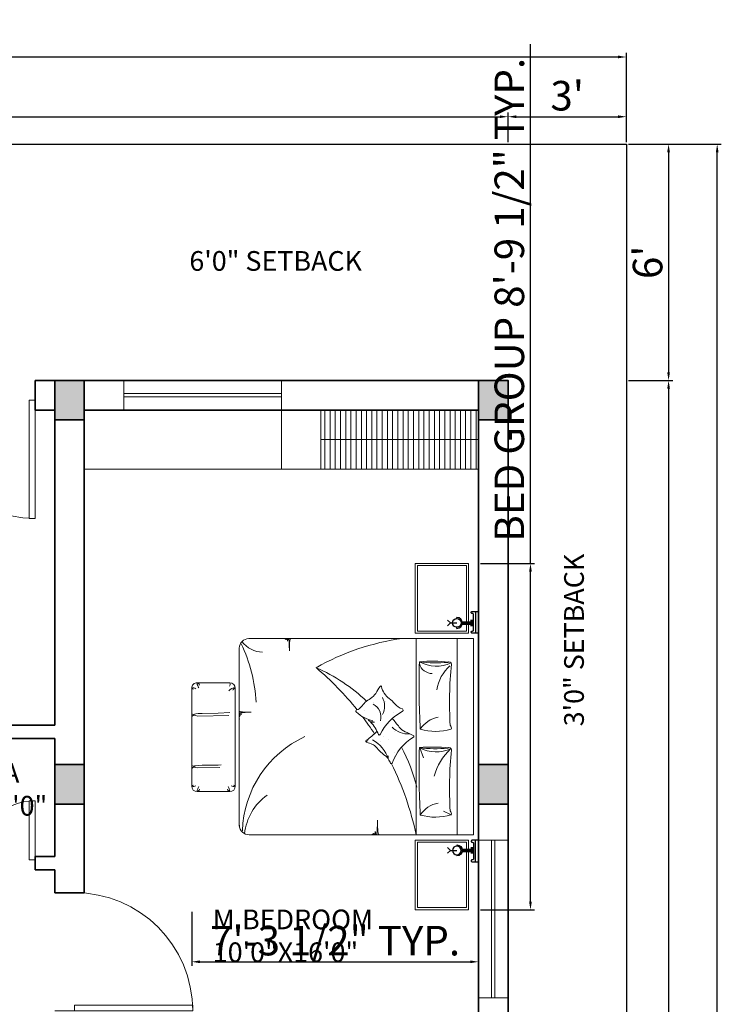
# Model space of a CAD drawing. Units: inches. Extents: x 3321 to 5237, y 11 to 1752.
# Tile 12 of 43: x 3652 to 3866, y 1445 to 1745. Entities that reach past the tile are written whole.
import ezdxf

# ---------------------------------------------------------------- set-up
doc = ezdxf.new("R2010")
doc.units = ezdxf.units.IN
for name, color, linetype, lineweight in [('A-ANNO-DIMS', 2, 'Continuous', 18), ('A-ANNO-TEXT', 7, 'Continuous', 18), ('A-AREA-IDEN', 7, 'Continuous', 18), ('A-COLS', 1, 'Continuous', 35), ('A-DOOR', 4, 'Continuous', 18), ('A-FLOR-CASE', 8, 'Continuous', 18), ('A-FLOR-CASE-PATT', 8, 'Continuous', 13), ('A-GLAZ', 5, 'Continuous', 18), ('A-WALL', 7, 'Continuous', 35), ('C-PROP', 7, 'Continuous', 30), ('FUR', 42, 'Continuous', 18)]:
    doc.layers.add(name, color=color, linetype=linetype, lineweight=lineweight)
for name, color, linetype in [('CEIL', 4, 'Continuous'), ('ELEC', 4, 'Continuous'), ('wood', 26, 'Continuous')]:
    doc.layers.add(name, color=color, linetype=linetype)
doc.styles.get("Standard").update_dxf_attribs({"font": 'arial.ttf'})
doc.dimstyles.new('ISO-25', dxfattribs={"dimtxt": 9, "dimasz": 2.5, "dimexe": 1.25, "dimexo": 0.625, "dimtad": 1, "dimdec": 1, "dimlunit": 3, "dimtxsty": 'Standard', "dimcen": 2.5, "dimclrd": 4, "dimclre": 4, "dimclrt": 256, "dimadec": 0, "dimazin": 0, "dimtfac": 1, "dimtdec": 1, "dimtmove": 0, "dimatfit": 3, "dimfxl": 1, "dimarcsym": 0})

# ---------------------------------------------------------------- blocks, each defined once
blk = doc.blocks.new('*U4')
for p, q in [((0, 0), (0, -6)), ((-36, 0), (-36, -6))]:
    blk.add_line(p, q)
blk.add_lwpolyline([(0, 0), (0, 36), (-1.75, 36), (-1.75, 0)], close=True)
blk.add_arc((0, 0), 36, 90, 180)
blk = doc.blocks.new('*U11')
for p, q in [((0, 0), (0, -6)), ((36, 0), (36, -6))]:
    blk.add_line(p, q)
blk.add_lwpolyline([(0, 0), (0, 36), (1.75, 36), (1.75, 0)], close=True)
blk.add_arc((0, 0), 36, 0, 90)
blk = doc.blocks.new('*D39')
at = {"layer": 'A-ANNO-DIMS', "color": 0, "lineweight": -2, "transparency": 16777216}
for p, q in [((3461.69, 1707.96), (3461.69, 1716.91)), ((3464.19, 1715.66), (3798.19, 1715.66)), ((3800.69, 1707.96), (3800.69, 1716.91))]:
    blk.add_line(p, q, dxfattribs=at)
at = {"layer": 'A-ANNO-DIMS', "color": 0, "transparency": 16777216}
for points in [[(3464.19, 1716.08), (3464.19, 1715.25), (3461.69, 1715.66)], [(3798.19, 1716.08), (3798.19, 1715.25), (3800.69, 1715.66)]]:
    blk.add_solid(points, dxfattribs=at)
at = {"layer": 'Defpoints', "color": 0, "transparency": 16777216}
for p in [(3800.69, 1715.66), (3461.69, 1707.34), (3800.69, 1707.34)]:
    blk.add_point(p, dxfattribs=at)
at = {"layer": 'A-ANNO-DIMS', "color": 0, "transparency": 16777216, "insert": (3631.19, 1720.89), "char_height": 9, "attachment_point": 5}
blk.add_mtext('28\'-3"', dxfattribs=at)
blk = doc.blocks.new('*D40')
at = {"layer": 'A-ANNO-DIMS', "color": 0, "lineweight": -2, "transparency": 16777216}
for p, q in [((3800.69, 1707.96), (3800.69, 1716.91)), ((3803.19, 1715.66), (3834.19, 1715.66)), ((3836.69, 1707.96), (3836.69, 1716.91))]:
    blk.add_line(p, q, dxfattribs=at)
at = {"layer": 'A-ANNO-DIMS', "color": 0, "transparency": 16777216}
for points in [[(3803.19, 1716.08), (3803.19, 1715.25), (3800.69, 1715.66)], [(3834.19, 1716.08), (3834.19, 1715.25), (3836.69, 1715.66)]]:
    blk.add_solid(points, dxfattribs=at)
at = {"layer": 'Defpoints', "color": 0, "transparency": 16777216}
for p in [(3836.69, 1715.66), (3800.69, 1707.34), (3836.69, 1707.34)]:
    blk.add_point(p, dxfattribs=at)
at = {"layer": 'A-ANNO-DIMS', "color": 0, "transparency": 16777216, "insert": (3818.69, 1720.89), "char_height": 9, "attachment_point": 5}
blk.add_mtext("3'", dxfattribs=at)
blk = doc.blocks.new('*D41')
at = {"layer": 'A-ANNO-DIMS', "color": 0, "lineweight": -2, "transparency": 16777216}
for p, q in [((3837.31, 1707.34), (3850.8, 1707.34)), ((3849.55, 1704.84), (3849.55, 1637.84)), ((3837.31, 1635.34), (3850.8, 1635.34))]:
    blk.add_line(p, q, dxfattribs=at)
at = {"layer": 'A-ANNO-DIMS', "color": 0, "transparency": 16777216}
for points in [[(3849.13, 1704.84), (3849.96, 1704.84), (3849.55, 1707.34)], [(3849.13, 1637.84), (3849.96, 1637.84), (3849.55, 1635.34)]]:
    blk.add_solid(points, dxfattribs=at)
at = {"layer": 'Defpoints', "color": 0, "transparency": 16777216}
for p in [(3836.69, 1707.34), (3836.69, 1635.34), (3849.55, 1635.34)]:
    blk.add_point(p, dxfattribs=at)
at = {"layer": 'A-ANNO-DIMS', "color": 0, "transparency": 16777216, "insert": (3844.33, 1671.34), "char_height": 9, "attachment_point": 5, "rotation": 90}
blk.add_mtext("6'", dxfattribs=at)
blk = doc.blocks.new('*D42')
at = {"layer": 'A-ANNO-DIMS', "color": 0, "lineweight": -2, "transparency": 16777216}
for p, q in [((3837.31, 1635.34), (3850.8, 1635.34)), ((3849.55, 1632.84), (3849.55, 1093.84)), ((3837.31, 1091.34), (3850.8, 1091.34))]:
    blk.add_line(p, q, dxfattribs=at)
at = {"layer": 'A-ANNO-DIMS', "color": 0, "transparency": 16777216}
for points in [[(3849.13, 1632.84), (3849.96, 1632.84), (3849.55, 1635.34)], [(3849.13, 1093.84), (3849.96, 1093.84), (3849.55, 1091.34)]]:
    blk.add_solid(points, dxfattribs=at)
at = {"layer": 'Defpoints', "color": 0, "transparency": 16777216}
for p in [(3836.69, 1635.34), (3836.69, 1091.34), (3849.55, 1091.34)]:
    blk.add_point(p, dxfattribs=at)
at = {"layer": 'A-ANNO-DIMS', "color": 0, "transparency": 16777216, "insert": (3844.35, 1363.34), "char_height": 9, "attachment_point": 5, "rotation": 90}
blk.add_mtext('45\'-4"', dxfattribs=at)
blk = doc.blocks.new('*D44')
at = {"layer": 'A-ANNO-DIMS', "color": 0, "lineweight": -2, "transparency": 16777216}
for p, q in [((3356.69, 1707.96), (3356.69, 1735.11)), ((3359.19, 1733.86), (3834.19, 1733.86)), ((3836.69, 1707.96), (3836.69, 1735.11))]:
    blk.add_line(p, q, dxfattribs=at)
at = {"layer": 'A-ANNO-DIMS', "color": 0, "transparency": 16777216}
for points in [[(3359.19, 1734.28), (3359.19, 1733.45), (3356.69, 1733.86)], [(3834.19, 1734.28), (3834.19, 1733.45), (3836.69, 1733.86)]]:
    blk.add_solid(points, dxfattribs=at)
at = {"layer": 'Defpoints', "color": 0, "transparency": 16777216}
for p in [(3836.69, 1733.86), (3356.69, 1707.34), (3836.69, 1707.34)]:
    blk.add_point(p, dxfattribs=at)
at = {"layer": 'A-ANNO-DIMS', "color": 0, "transparency": 16777216, "insert": (3596.69, 1739.08), "char_height": 9, "attachment_point": 5}
blk.add_mtext("40'", dxfattribs=at)
blk = doc.blocks.new('*D47')
at = {"layer": 'A-ANNO-DIMS', "color": 0, "lineweight": -2, "transparency": 16777216}
for p, q in [((3837.31, 1707.34), (3865.6, 1707.34)), ((3864.35, 989.84), (3864.35, 1704.84)), ((3837.31, 987.34), (3865.6, 987.34))]:
    blk.add_line(p, q, dxfattribs=at)
at = {"layer": 'A-ANNO-DIMS', "color": 0, "transparency": 16777216}
for points in [[(3863.93, 1704.84), (3864.76, 1704.84), (3864.35, 1707.34)], [(3863.93, 989.84), (3864.76, 989.84), (3864.35, 987.34)]]:
    blk.add_solid(points, dxfattribs=at)
at = {"layer": 'Defpoints', "color": 0, "transparency": 16777216}
for p in [(3836.69, 1707.34), (3864.35, 1707.34), (3836.69, 987.34)]:
    blk.add_point(p, dxfattribs=at)
at = {"layer": 'A-ANNO-DIMS', "color": 0, "transparency": 16777216, "insert": (3859.13, 1347.34), "char_height": 9, "attachment_point": 5, "rotation": 90}
blk.add_mtext("60'", dxfattribs=at)
blk = doc.blocks.new('*X127')
at = {"color": 0}
for p, q in [((3147.8, 8143.4), (3147.8, 8143.4)), ((3155.9, 8182.9), (3155.9, 8182.9)), ((3283, 8049.6), (3283, 8049.6)), ((3209.5, 8023.9), (3209.5, 8023.9)), ((3251.6, 7997), (3251.6, 7997)), ((3154.1, 7950.7), (3154.1, 7950.7))]:
    blk.add_line(p, q, dxfattribs=at)
blk = doc.blocks.new('*X126')
at = {"color": 0}
for p, q in [((3155.9, 8182.9), (3155.9, 8182.9)), ((3139.8, 7939.7), (3139.8, 7939.7))]:
    blk.add_line(p, q, dxfattribs=at)
blk = doc.blocks.new('*X125')
at = {"color": 0}
for p, q in [((3155.9, 8182.9), (3155.9, 8182.9)), ((3139.8, 7939.7), (3139.8, 7939.7))]:
    blk.add_line(p, q, dxfattribs=at)
blk = doc.blocks.new('*X124')
at = {"color": 0}
for p, q in [((3163, 7776.2), (3163, 7776.2)), ((3244.3, 7698.6), (3244.3, 7698.6)), ((3340.3, 7689.4), (3340.3, 7689.4)), ((3422.2, 7761.3), (3422.2, 7761.3)), ((3236.2, 7675.7), (3236.2, 7675.7))]:
    blk.add_line(p, q, dxfattribs=at)
blk = doc.blocks.new('BED1')
for p, q in [((0, -1000), (0, 800)), ((150, 800), (0, 800)), ((150, 800), (150, -1000)), ((2058.7, 800), (150, 800)), ((528, 800), (528, -1000)), ((211.8, 614.9), (277.5, 585.4)), ((2537.2, 404.9), (2237.2, 404.9)), ((2187.2, 354.9), (2187.2, -545.1)), ((2587.2, -545.1), (2587.2, 354.9)), ((2582, 188.1), (2565.4, 174.8)), ((2566.3, 178.5), (2565.2, 177.4)), ((2565.4, 174.8), (2585.7, 165.4)), ((2566.3, -296.8), (2565.2, -297.9)), ((2582, -287.1), (2565.4, -300.5)), ((2565.4, -300.5), (2585.7, -309.9)), ((2237.2, -595.1), (2537.2, -595.1)), ((150, -1000), (0, -1000)), ((150, -1000), (2063.5, -1000))]:
    blk.add_line(p, q)
for points in [[(934, 797.9), (930.9, 797.7), (928.3, 797.4), (926.3, 796.9), (924.9, 796.3), (923.8, 795.6), (923.1, 794.8), (922.7, 793.8), (922.5, 792.7), (922.4, 791.5), (922.5, 790.3), (922.6, 789.2), (922.6, 788.3), (922.6, 787.6), (922.4, 787.3), (922, 787.4), (921.4, 787.9), (920.6, 788.9), (919.5, 790.2), (918.4, 791.6), (917.1, 793.1), (915.9, 794.6), (914.6, 796), (913.3, 797.1), (912.2, 797.9), (911.1, 798.3), (910.1, 798.4), (909.2, 798), (908.3, 797.1), (907.5, 795.8), (906.8, 793.9), (906, 791.4), (905.4, 788.5), (904.8, 785.2), (904.2, 781.7), (903.7, 778.4), (903.2, 775.4), (902.8, 772.9), (902.5, 771.3), (902.3, 770.6), (902.1, 771.2), (902, 772.8), (901.8, 775.2), (901.7, 778.1), (901.5, 781.5), (901.2, 785), (900.8, 788.4), (900.2, 791.5), (899.5, 794.1), (898.6, 796.2), (897.6, 797.9), (896.5, 799.2), (895.3, 800), (894.1, 800.5), (893, 800.7), (891.9, 800.5), (890.9, 800.1), (890, 799), (889.1, 797.1), (888.3, 794), (887.6, 789.3), (886.9, 782.9), (886.2, 774.2), (885.5, 763.1), (884.8, 749.5), (884.2, 734.2), (883.6, 718.3), (883, 702.8), (882.5, 688.8), (882, 677.5), (881.7, 669.8), (881.5, 666.9), (881.3, 669.4), (881.3, 676.7), (881.3, 687.8), (881.2, 701.5), (881.1, 716.8), (880.8, 732.6), (880.2, 748), (879.4, 761.8), (878.3, 773.2), (876.9, 782.2), (875.1, 789.2), (872.9, 794.4), (870.3, 798), (869, 799)], [(2150, -913.5), (2150, 723.2)], [(2327.6, 182.3), (2530, 185.9), (2550.8, 181.9), (2561.7, 179), (2566, 176.7), (2566.9, 174.4), (2566.3, 171.9), (2562, 169.2), (2550.3, 166.5), (2527.7, 163.9), (2490.6, 161.8), (2345.5, 160.2), (2317.8, 158.5)], [(494.7, 3.1), (458.9, 95.3)], [(2149.7, -259.9), (2150, -268.4), (2150.1, -274.1), (2150.1, -278.1), (2150, -281.4), (2149.8, -284), (2149.5, -286.1), (2149.1, -287.8), (2148.7, -289), (2148.1, -289.9), (2147.4, -290.5), (2146.6, -290.8), (2145.6, -291), (2144.6, -291), (2143.6, -291), (2142.7, -290.9), (2141.9, -290.9), (2141.4, -290.9), (2141.1, -291), (2141.2, -291.4), (2141.7, -291.9), (2142.5, -292.6), (2143.5, -293.4), (2144.7, -294.4), (2146, -295.4), (2147.2, -296.5), (2148.4, -297.6), (2149.3, -298.6), (2150, -299.6), (2150.3, -300.5), (2150.4, -301.3), (2150, -302.1), (2149.3, -302.8), (2148.2, -303.5), (2146.6, -304.1), (2144.6, -304.7), (2142.1, -305.2), (2139.3, -305.7), (2136.5, -306.2), (2133.7, -306.6), (2131.2, -307), (2129.2, -307.3), (2127.8, -307.6), (2127.3, -307.8), (2127.7, -308), (2129, -308.1), (2131, -308.2), (2133.5, -308.3), (2136.3, -308.5), (2139.2, -308.7), (2142, -309), (2144.6, -309.5), (2146.8, -310.1), (2148.6, -310.9), (2150, -311.7), (2151, -312.7), (2151.7, -313.6), (2152.1, -314.6), (2152.3, -315.6), (2152.2, -316.5), (2151.8, -317.3), (2150.9, -318.1), (2149.3, -318.8), (2146.7, -319.4), (2142.8, -320), (2137.4, -320.6), (2130.2, -321.2), (2121, -321.8), (2109.7, -322.3), (2096.9, -322.9), (2083.6, -323.4), (2070.7, -323.9), (2059.1, -324.3), (2049.6, -324.7), (2043.2, -325), (2040.8, -325.2), (2042.9, -325.3), (2049, -325.3), (2058.2, -325.3), (2069.6, -325.4), (2082.3, -325.5), (2095.6, -325.8), (2108.4, -326.2), (2119.9, -326.8), (2129.4, -327.8), (2136.9, -329), (2142.7, -330.5), (2147, -332.3), (2150, -334.4), (2150.9, -335.6)], [(2246.5, -294.4), (2530, -289.4), (2550.8, -293.4), (2561.7, -296.3), (2566, -298.6), (2566.9, -300.8), (2566.3, -303.4), (2562, -306.1), (2550.3, -308.8), (2527.7, -311.3), (2490.6, -313.5), (2345.5, -315), (2238.6, -321.8)], [(1733.7, -998.3), (1731.1, -998.1), (1729, -997.8), (1727.4, -997.4), (1726.1, -997), (1725.2, -996.4), (1724.7, -995.7), (1724.3, -994.8), (1724.1, -993.9), (1724.1, -992.9), (1724.1, -991.9), (1724.2, -991), (1724.2, -990.2), (1724.2, -989.7), (1724.1, -989.4), (1723.8, -989.5), (1723.2, -990), (1722.5, -990.8), (1721.7, -991.8), (1720.7, -993), (1719.7, -994.3), (1718.6, -995.5), (1717.5, -996.6), (1716.5, -997.6), (1715.5, -998.3), (1714.6, -998.6), (1713.8, -998.6), (1713, -998.3), (1712.3, -997.6), (1711.7, -996.5), (1711, -994.9), (1710.4, -992.9), (1709.9, -990.4), (1709.4, -987.6), (1708.9, -984.8), (1708.5, -982), (1708.1, -979.5), (1707.8, -977.4), (1707.5, -976.1), (1707.3, -975.5), (1707.1, -976), (1707, -977.3), (1706.9, -979.3), (1706.8, -981.8), (1706.7, -984.6), (1706.4, -987.5), (1706.1, -990.3), (1705.6, -992.9), (1705, -995.1), (1704.2, -996.9), (1703.4, -998.3), (1702.4, -999.3), (1701.5, -1000), (1700.5, -1000.4), (1699.6, -1000.6), (1698.7, -1000.4), (1697.8, -1000.1), (1697, -999.2), (1696.3, -997.6), (1695.7, -995), (1695.1, -991.1), (1694.5, -985.7), (1693.9, -978.5), (1693.3, -969.3), (1692.8, -957.9), (1692.2, -945.2), (1691.7, -931.9), (1691.2, -919), (1690.8, -907.4), (1690.4, -897.9), (1690.1, -891.5), (1689.9, -889.1), (1689.8, -891.2), (1689.8, -897.3), (1689.8, -906.5), (1689.7, -917.9), (1689.6, -930.6), (1689.4, -943.8), (1688.9, -956.6), (1688.3, -968.1), (1687.3, -977.6), (1686.1, -985.2), (1684.6, -991), (1682.8, -995.3), (1680.7, -998.3), (1679.6, -999.2)]]:
    blk.add_lwpolyline(points)
for points in [[(489.2, 619.6, 0.144019), (207.6, 617.9, 0.248643)], [(205.5, 619.6, 0.267769), (215.1, 582.4, -0.037739), (204.3, 21.8, 0.684696), (236.7, 5.5, -0.060702), (497.2, 0.1, -0.046649), (225.9, 3.1, -1.318436)], [(497.2, 0.1, 0.021276), (489.2, 619.6, -0.206383), (326.6, 509.4, 0.237198)], [(211.8, 12.8, 0.143972), (361.6, 262.9, 1.292232)], [(886.4, -150, -0.069098), (985, -66.5, 0.658965), (982.1, -48.7, -0.049789), (927.4, -29, -0.103757), (896.6, -5.4, 0.055725), (800.9, 83.3, -0.11866), (782.7, 104.9, 0.016811), (761.6, 143.9, 0.70791), (748.3, 144, -0.16964), (551.9, -96.6, 0.664036), (554, -110.7, 0.023706), (627, -144.7, -0.134834), (683.2, -188, 0.012748), (746.3, -267.4)], [(205.5, -168.2, 0.267769), (215.1, -205.4, -0.037739), (204.3, -766, 0.684696), (236.7, -782.3, -0.060702), (497.2, -787.7, -0.046649), (225.9, -784.7, -1.318436)], [(489.2, -168.2, 0.144019), (207.6, -169.9, 0.248643)], [(497.2, -787.7, 0.021276), (489.2, -168.2, -0.206383), (326.6, -278.4, 0.237198)], [(969.1, -259.1, 0.263265), (936.3, -236.9, -0.026108), (909.2, -233.2, 0.027613), (945.1, -234.2, -0.089259), (872.7, -120, 0.662242), (857.6, -119.3, -0.162037), (651.8, -332.7, 0.676499), (654, -354.5, -0.160513), (722.9, -401.5, 0.07473), (773.5, -450.3, -0.187721), (845.5, -559.9, 0.70791), (858.8, -561.4, -0.010003), (898.6, -497.3, -0.113819), (947.3, -450.2, 0.099539), (1032.5, -372.4, -0.173425), (1070.9, -346.4, 0.589988), (1076.2, -326.1, 0.137312), (923.9, -245.9, 0.137312)], [(1446, -733.4, -0.095039), (652.8, -1001.7)]]:
    blk.add_lwpolyline(points, format="xyb")
for centre, radius, start, end in [((3208.8, 1363.3), 2739.4, 191.86791, 206.32469), ((1138.6, 793.9), 983.2, 294.60777, 358.30329), ((1608.1, 842.5), 496.3, 305.19014, 354.02057), ((2062.7, 713.7), 86.5, 0, 93.53765), ((2098.7, 754.7), 1625, 193.90497, 207.81692), ((2237.2, 354.9), 50, 90, 180), ((2321.1, 409.7), 84.5, 185.61958, 217.13957), ((2227.5, 373.5), 32.8, 17.83305, 72.80048), ((2546.9, 373.5), 32.8, 107.19952, 162.16695), ((2453.3, 409.7), 84.5, 322.86043, 354.38042), ((2537.2, 354.9), 50, 0, 90), ((2201.9, 323.3), 34.8, 50.8413, 114.9586), ((2212.2, 381.5), 36.5, 226.80948, 258.3841), ((2572.5, 323.3), 34.8, 65.0414, 129.1587), ((2562.2, 381.5), 36.5, 281.6159, 313.19052), ((751.8, 88.7), 34.9, 336.83517, 27.72181), ((684.2, 86), 100.3, 353.675, 10.88198), ((1074.1, 198.8), 306.1, 197.86019, 241.51221), ((341.4, -277.7), 318.5, 60.71255, 115.00895), ((983.7, -79.5), 20.8, 73.79673, 130.45661), ((978.5, -68.6), 14.3, 39.7097, 85.9506), ((602.5, -324), 198.6, 43.20348, 95.05559), ((3208.8, 1363.3), 2739.4, 212.93136, 216.95099), ((981.1, -281.8), 131.1, 164.0372, 243.45361), ((980, -379), 163.4, 152.61037, 209.36102), ((3208.8, 1363.3), 2739.4, 218.63292, 229.94485), ((2098.7, 754.7), 1625, 226.58872, 246.3156), ((3402.5, -342.9), 1408.5, 182.99169, 205.68187), ((-34.4, -471.2), 376.5, 312.01178, 350.96348), ((2178, -513.5), 33, 286.18268, 338.13858), ((2188.1, -476.2), 73, 269.45125, 322.80265), ((2572.5, -513.6), 34.8, 230.8413, 294.9586), ((2562.2, -571.8), 36.5, 46.80948, 78.3841), ((2237.2, -545.1), 50, 180, 270), ((2271.1, -580.9), 35.8, 148.90546, 197.55407), ((2546.9, -563.8), 32.8, 197.83305, 252.80048), ((2453.3, -600), 84.5, 5.61958, 37.13957), ((2537.2, -545.1), 50, 270, 0), ((375.7, -807.4), 128.2, 17.40732, 88.51286), ((341.4, -1065.5), 318.5, 60.71255, 115.00895), ((1929.1, -1126), 250.5, 37.85533, 88.44053), ((2063.5, -913.5), 86.5, 270, 0)]:
    blk.add_arc(centre, radius, start, end)
for name in ['*X126', '*X125', '*X127', '*X124']:
    blk.add_blockref(name, (-2425.3, -8101.4))
blk = doc.blocks.new('APLIQ')
at = {"layer": 'ELEC'}
for p, q in [((0, 0.2), (-0.0261, 0.2261)), ((0, 0.2), (0.0261, 0.2261)), ((0, 0.2), (0, 0.14)), ((-0.05, 0.14), (-0.04, 0.14)), ((0.04, 0.14), (0.05, 0.14)), ((-0.03, 0.01), (0.03, 0.01)), ((-0.03, 0), (0.03, 0)), ((-0.01, 0.09), (-0.01, 0.01)), ((0, 0.09), (0, 0)), ((0.01, 0.09), (0.01, 0.01))]:
    blk.add_line(p, q, dxfattribs=at)
blk.add_circle((0, 0.14), 0.04, dxfattribs=at)
blk.add_arc((0, 0.14), 0.05, 180, 0, dxfattribs=at)
blk = doc.blocks.new('A$C68AE1801')
at = {"layer": 'FUR'}
for points in [[(2.5416, 3.18), (2.5416, 2.54), (2.0516, 2.54), (2.0516, 3.18)], [(2.5216, 3.16), (2.5216, 2.56), (2.0716, 2.56), (2.0716, 3.16)], [(2.5416, 0), (2.5416, 0.64), (2.0516, 0.64), (2.0516, 0)], [(2.5216, 0.02), (2.5216, 0.62), (2.0716, 0.62), (2.0716, 0.02)]]:
    blk.add_lwpolyline(points, close=True, dxfattribs=at)
at = {"layer": 'wood'}
for p, q in [((2.6057, 2.74), (2.6057, 2.54)), ((2.6057, 0.44), (2.6057, 0.64))]:
    blk.add_line(p, q, dxfattribs=at)
for points in [[(2.5657, 2.728), (2.5657, 2.732, -0.414214), (2.5737, 2.74), (2.6321, 2.74), (2.6321, 2.54), (2.5737, 2.54, -0.414214), (2.5657, 2.548), (2.5657, 2.552, -0.414214), (2.5737, 2.56), (2.5777, 2.56, 0.414214), (2.5857, 2.568), (2.5857, 2.712, 0.414214), (2.5777, 2.72), (2.5737, 2.72, -0.414214)], [(2.5657, 0.452), (2.5657, 0.448, 0.414214), (2.5737, 0.44), (2.6321, 0.44), (2.6321, 0.64), (2.5737, 0.64, 0.414214), (2.5657, 0.632), (2.5657, 0.628, 0.414214), (2.5737, 0.62), (2.5777, 0.62, -0.414214), (2.5857, 0.612), (2.5857, 0.468, -0.414214), (2.5777, 0.46), (2.5737, 0.46, 0.414214)]]:
    blk.add_lwpolyline(points, format="xyb", close=True, dxfattribs=at)
at = {"layer": 'CEIL', "rotation": 90}
blk.add_blockref('APLIQ', (2.5736, 2.634), dxfattribs=at)
at = {"layer": 'CEIL', "xscale": -1, "rotation": 90}
blk.add_blockref('APLIQ', (2.5736, 0.546), dxfattribs=at)
at = {"layer": 'FUR', "xscale": 0.001, "yscale": 0.001, "zscale": 0.001, "rotation": 180}
blk.add_blockref('BED1', (2.5872, 1.49), dxfattribs=at)
blk = doc.blocks.new('COL-9X12-FURN-PLAN')
h = blk.add_hatch(color=256)
h.dxf.hatch_style = 1
h.paths.add_polyline_path([(0, 12), (0, 0), (9, 0), (9, 12)])
blk.add_lwpolyline([(0, 0), (9, 0), (9, 12), (0, 12)], close=True)
blk = doc.blocks.new('WIN-48IN-9IN-WALL')
for p, q in [((0, 0), (0, 9)), ((48, 0), (48, 9)), ((0, 5), (48, 5)), ((0, 4), (48, 4))]:
    blk.add_line(p, q)
blk = doc.blocks.new('DOOR-DOUBLE-36IN')
for p, q in [((0, 3), (0, 0)), ((18, 3), (18, 0)), ((18, 3), (18, 0)), ((36, 3), (36, 0))]:
    blk.add_line(p, q)
for points in [[(0, 3), (0, 21), (1.75, 21), (1.75, 3)], [(36, 3), (36, 21), (34.25, 21), (34.25, 3)]]:
    blk.add_lwpolyline(points, close=True)
for centre, start, end in [((0, 3), 0, 90), ((36, 3), 90, 180)]:
    blk.add_arc(centre, 18, start, end)
blk = doc.blocks.new('PROPERTY-40X60FT')
for p, q in [((0, 720), (480, 720)), ((480, 720), (480, 0))]:
    blk.add_line(p, q)
blk = doc.blocks.new('*D191')
at = {"layer": 'A-ANNO-DIMS', "color": 4, "lineweight": -2, "transparency": 16777216}
for p, q in [((3807.51, 1579.6), (3807.51, 1737.72)), ((3792.31, 1579.6), (3808.76, 1579.6)), ((3807.51, 1476.61), (3807.51, 1577.1)), ((3792.31, 1474.11), (3808.76, 1474.11))]:
    blk.add_line(p, q, dxfattribs=at)
at = {"layer": 'A-ANNO-DIMS', "color": 4, "transparency": 16777216}
for points in [[(3807.09, 1577.1), (3807.93, 1577.1), (3807.51, 1579.6)], [(3807.09, 1476.61), (3807.93, 1476.61), (3807.51, 1474.11)]]:
    blk.add_solid(points, dxfattribs=at)
at = {"layer": 'Defpoints', "color": 0, "transparency": 16777216}
for p in [(3791.69, 1579.6), (3807.51, 1579.6), (3791.69, 1474.11)]:
    blk.add_point(p, dxfattribs=at)
at = {"layer": 'A-ANNO-DIMS', "transparency": 16777216, "insert": (3802.23, 1659.91), "char_height": 9, "attachment_point": 5, "rotation": 90}
blk.add_mtext('BED GROUP 8\'-9 1/2" TYP.', dxfattribs=at)
blk = doc.blocks.new('*D192')
at = {"layer": 'A-ANNO-DIMS', "color": 4, "lineweight": -2, "transparency": 16777216}
for p, q in [((3704.38, 1473.48), (3704.38, 1457.04)), ((3791.69, 1473.48), (3791.69, 1457.04)), ((3706.88, 1458.29), (3789.19, 1458.29))]:
    blk.add_line(p, q, dxfattribs=at)
at = {"layer": 'A-ANNO-DIMS', "color": 4, "transparency": 16777216}
for points in [[(3706.88, 1458.7), (3706.88, 1457.87), (3704.38, 1458.29)], [(3789.19, 1458.7), (3789.19, 1457.87), (3791.69, 1458.29)]]:
    blk.add_solid(points, dxfattribs=at)
at = {"layer": 'Defpoints', "color": 0, "transparency": 16777216}
for p in [(3704.38, 1474.11), (3791.69, 1474.11), (3791.69, 1458.29)]:
    blk.add_point(p, dxfattribs=at)
at = {"layer": 'A-ANNO-DIMS', "transparency": 16777216, "insert": (3748.03, 1463.57), "char_height": 9, "attachment_point": 5}
blk.add_mtext('7\'-3 1/2" TYP.', dxfattribs=at)

msp = doc.modelspace()

# ---------------------------------------------------------------- hatches: boundary and pattern name
at = {"layer": 'A-FLOR-CASE-PATT'}
h = msp.add_hatch(dxfattribs=at)
h.set_pattern_fill('ANSI31', color=256, scale=0.5, angle=45)
h.paths.add_polyline_path([(3791.69, 1626.34), (3743.69, 1626.34), (3743.69, 1608.34), (3791.69, 1608.34)])

# ---------------------------------------------------------------- linework, layer by layer
at = {"layer": 'A-FLOR-CASE'}
for p, q in [((3731.69, 1626.34), (3731.69, 1608.34)), ((3743.69, 1626.34), (3743.69, 1608.34)), ((3743.69, 1617.34), (3791.69, 1617.34)), ((3671.69, 1608.34), (3791.69, 1608.34))]:
    msp.add_line(p, q, dxfattribs=at)
at = {"layer": 'A-WALL'}
for p, q in [((3656.69, 1635.34), (3656.69, 1626.34)), ((3656.69, 1635.34), (3800.69, 1635.34)), ((3800.69, 1635.34), (3800.69, 1091.34)), ((3656.69, 1626.34), (3662.69, 1626.34)), ((3662.69, 1626.34), (3662.69, 1530.34)), ((3671.69, 1626.34), (3671.69, 1479.34)), ((3671.69, 1626.34), (3791.69, 1626.34)), ((3791.69, 1626.34), (3791.69, 1434.34)), ((3577.69, 1530.34), (3662.69, 1530.34)), ((3614.69, 1526.34), (3662.69, 1526.34)), ((3662.69, 1526.34), (3662.69, 1490.34)), ((3656.69, 1490.34), (3656.69, 1486.34)), ((3656.69, 1490.34), (3662.69, 1490.34)), ((3656.69, 1486.34), (3662.69, 1486.34)), ((3662.69, 1486.34), (3662.69, 1479.34)), ((3662.69, 1479.34), (3671.69, 1479.34))]:
    msp.add_line(p, q, dxfattribs=at)

# ---------------------------------------------------------------- block references
at = {"layer": 'A-COLS'}
for p in [(3662.69, 1623.34), (3791.69, 1623.34), (3662.69, 1506.34), (3791.69, 1506.34)]:
    msp.add_blockref('COL-9X12-FURN-PLAN', p, dxfattribs=at)
at = {"layer": 'A-DOOR'}
for name, p, rotation in [('*U11', (3656.69, 1629.34), 180), ('*U4', (3668.69, 1443.34), 270)]:
    msp.add_blockref(name, p, dxfattribs=dict(at, rotation=rotation))
msp.add_blockref('DOOR-DOUBLE-36IN', (3620.69, 1486.34), dxfattribs=at)
at = {"layer": 'A-GLAZ'}
msp.add_blockref('WIN-48IN-9IN-WALL', (3683.69, 1626.34), dxfattribs=at)
at = {"layer": 'A-GLAZ', "rotation": 89.9999999999993}
msp.add_blockref('WIN-48IN-9IN-WALL', (3800.69, 1447.34), dxfattribs=at)
at = {"layer": 'C-PROP'}
msp.add_blockref('PROPERTY-40X60FT', (3356.69, 987.34), dxfattribs=at)
at = {"layer": 'FUR', "xscale": 33.17188472218209, "yscale": 33.17188472218209, "zscale": 33.17188472218209}
msp.add_blockref('A$C68AE1801', (3704.38, 1474.11), dxfattribs=at)

# ---------------------------------------------------------------- texts
at = {"layer": 'A-ANNO-TEXT', "insert": (3703.67, 1674.74), "char_height": 6, "attachment_point": 1}
msp.add_mtext_dynamic_manual_height_columns('6\'0" SETBACK', width=97.3114, gutter_width=25, heights=[0], dxfattribs=at)
at = {"layer": 'A-ANNO-TEXT', "insert": (3817.76, 1530.01), "char_height": 6, "attachment_point": 1, "rotation": 90}
msp.add_mtext_dynamic_manual_height_columns('3\'0" SETBACK', width=97.3114, gutter_width=25, heights=[0], dxfattribs=at)
at = {"layer": 'A-AREA-IDEN', "char_height": 6, "attachment_point": 1}
for s, insert in [('POOJA\\P4\'0"X3\'0"', (3625.25, 1518.81)), ('M.BEDROOM\\P10\'0"X16\'0"', (3710.8, 1474.19))]:
    msp.add_mtext_dynamic_manual_height_columns(s, width=97.3114, gutter_width=25, heights=[0], dxfattribs=dict(at, insert=insert))

# ---------------------------------------------------------------- dimensions: what is measured, and where the dimension line sits
at = {"layer": 'A-ANNO-DIMS'}
for base, p1, p2, override, picture, middle in [((3836.69, 1733.86), (3356.69, 1707.34), (3836.69, 1707.34), {"dimclrd": 0, "dimclre": 0, "dimclrt": 0}, '*D44', (3596.69, 1739.08)), ((3800.69, 1715.66), (3461.69, 1707.34), (3800.69, 1707.34), {"dimclrd": 0, "dimclre": 0, "dimclrt": 0, "dimtmove": 1}, '*D39', (3631.19, 1720.89)), ((3836.69, 1715.66), (3800.69, 1707.34), (3836.69, 1707.34), {"dimclrd": 0, "dimclre": 0, "dimclrt": 0, "dimtmove": 1}, '*D40', (3818.69, 1720.89))]:
    dim = msp.add_linear_dim(base=base, p1=p1, p2=p2, dimstyle='ISO-25', override=override, dxfattribs=at)
    dim.commit()
    dim.dimension.update_dxf_attribs({"geometry": picture, "text_midpoint": middle})
dim = msp.add_linear_dim(base=(3807.51, 1579.6), p1=(3791.69, 1474.11), p2=(3791.69, 1579.6), angle=90, text='BED GROUP <> TYP.', dimstyle='ISO-25', override={"dimdec": 1, "dimlfac": 1, "dimrnd": 0, "dimzin": 1, "dimdsep": 46, "dimlunit": 4, "dimfrac": 2}, dxfattribs=at)
dim.commit()
dim.dimension.update_dxf_attribs({"geometry": '*D191', "text_midpoint": (3802.23, 1659.91)})
for base, p1, p2, angle, override, picture, middle in [((3849.55, 1635.34), (3836.69, 1707.34), (3836.69, 1635.34), 90, {"dimclrd": 0, "dimclre": 0, "dimclrt": 0}, '*D41', (3844.33, 1671.34)), ((3864.35, 1707.34), (3836.69, 987.34), (3836.69, 1707.34), 270, {"dimclrd": 0, "dimclre": 0, "dimclrt": 0}, '*D47', (3859.13, 1347.34)), ((3849.55, 1091.34), (3836.69, 1635.34), (3836.69, 1091.34), 90, {"dimclrd": 0, "dimclre": 0, "dimclrt": 0, "dimtmove": 1}, '*D42', (3844.35, 1363.34))]:
    dim = msp.add_linear_dim(base=base, p1=p1, p2=p2, angle=angle, dimstyle='ISO-25', override=override, dxfattribs=at)
    dim.commit()
    dim.dimension.update_dxf_attribs({"geometry": picture, "text_midpoint": middle})
dim = msp.add_linear_dim(base=(3791.69, 1458.29), p1=(3704.38, 1474.11), p2=(3791.69, 1474.11), text='<> TYP.', dimstyle='ISO-25', override={"dimdec": 1, "dimlfac": 1, "dimrnd": 0, "dimzin": 1, "dimdsep": 46, "dimlunit": 4, "dimfrac": 2}, dxfattribs=at)
dim.commit()
dim.dimension.update_dxf_attribs({"geometry": '*D192', "text_midpoint": (3748.03, 1463.57)})

doc.saveas('drawing.dxf')
